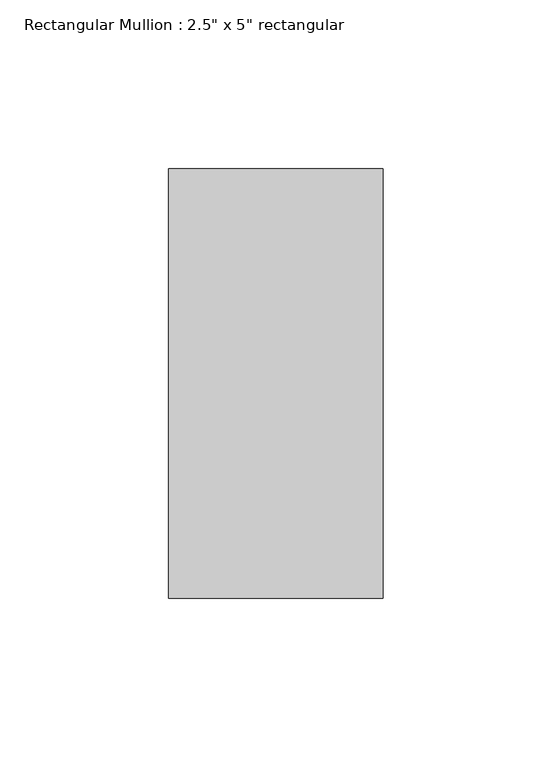
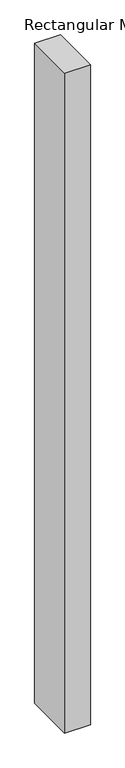
"""IFC4 building model written with IfcOpenShell, lengths in millimetres: member geometry."""

from ifc_helpers import new_model, si_unit, frame, origin, place, context, project, spatial, polyline, outline, extrude, source, transform, mapped, element, save


def member_5d841d64(model_context):
    return source(origin(), model_context, "Body", "SweptSolid", [
        extrude(outline(polyline([(0.0, 63.5), (0.0, -63.5), (-63.5, -63.5), (-63.5, 63.5), (0.0, 63.5)])), frame((0.0, 0.0, -1717.1019301), z_axis=(0.0, 0.0, 1.0), x_axis=(1.0, 0.0, 0.0)), (0.0, 0.0, 1.0), 1717.1019301),
    ])


if __name__ == "__main__":
    model = new_model("IFC4")
    model_context = context("Model", 3, world=origin())
    ifc_project = project(units=[si_unit("LENGTHUNIT", "METRE", prefix="MILLI")], contexts=[model_context])
    site = spatial("IfcSite", under=ifc_project)
    building = spatial("IfcBuilding", under=site)
    placement = place(None, origin())
    member_shape = member_5d841d64(model_context)
    element("IfcMember", 1, ObjectType="Rectangular Mullion : 2.5\" x 5\" rectangular", at=placement, inside=building, context=model_context, shape_type="MappedRepresentation", body=[
        mapped(member_shape, transform((0.0, 0.0, 0.0), x_axis=(1.0, 0.0, 0.0), y_axis=(0.0, 1.0, 0.0), z_axis=(0.0, 0.0, 1.0))),
    ])
    save(model, "model.ifc")

# Revit data of these elements
# Type "Rectangular Mullion : 2.5\" x 5\" rectangular"
#   built-in parameter 1007304 = 0.416667 (stored number, unit not read)
#   built-in parameter 1007301 = 0.104167 (stored number, unit not read)
#   built-in parameter 1007300 = 0.104167 (stored number, unit not read)
# Element 1 (IfcMember, "Rectangular Mullion : 2.5\" x 5\" rectangular")
#   Materials on its faces: "Aluminum"
# Materials
#   "Aluminum": class "Metal", colour RGB 247 247 247, transparency 0, Description = "Aluminum 6061", Cost = 0
